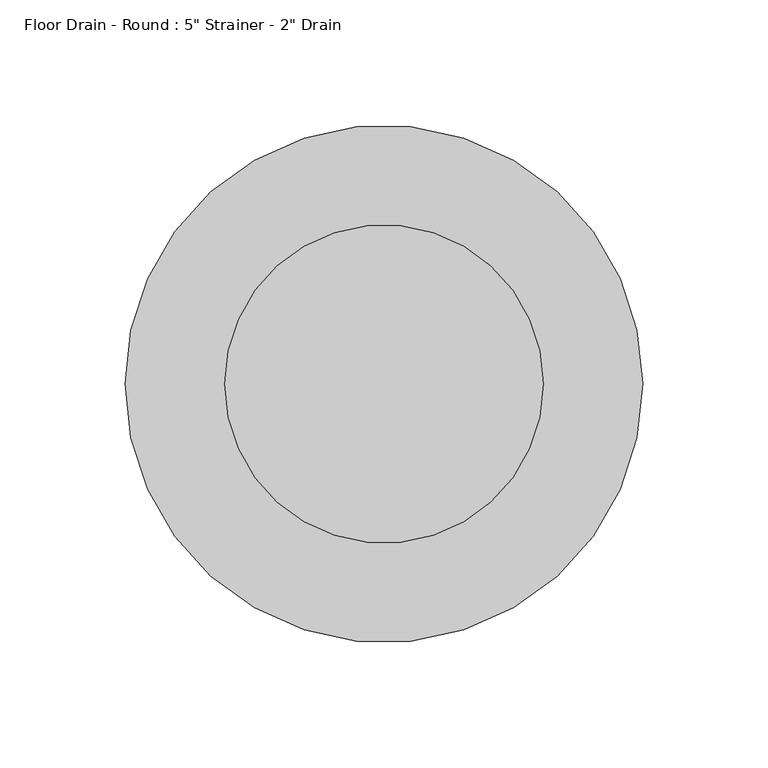
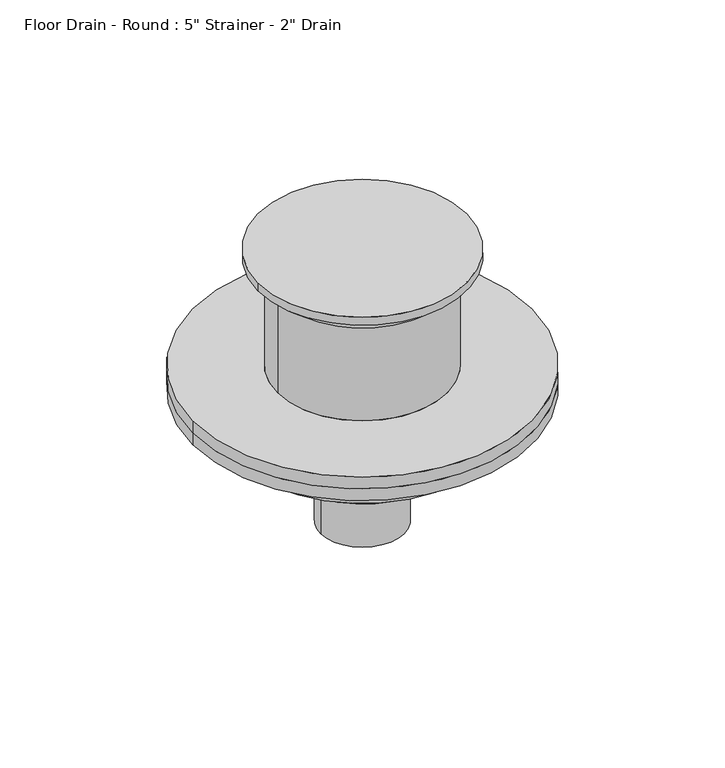
"""IFC4 building model written with IfcOpenShell, lengths in millimetres: flow terminal geometry."""

from ifc_helpers import new_model, si_unit, frame, origin, place, context, project, spatial, polyline, circle_curve, source, transform, mapped, element, save
from ifc_brep_helpers import plane_surface, cylinder_surface, revolved_surface, advanced_brep


def flow_terminal_accce45a(model_context):
    return source(origin(), model_context, "Body", "AdvancedBrep", [
        advanced_brep(
        [(103.1875, 0.0, -74.93), (-103.1875, 0.0, -74.93), (-51.59375, 0.0, -74.93), (51.59375, 0.0, -74.93), (103.1875, 0.0, -82.55), (-103.1875, 0.0, -82.55), (51.59375, 0.0, -15.24), (-51.59375, 0.0, -15.24), (-63.5, 0.0, -5.08), (63.5, 0.0, -5.08), (63.5, 0.0, 0.0), (-63.5, 0.0, 0.0)],
        [
            (0, 1, circle_curve(frame((0.0, 0.0, -74.93), z_axis=(0.0, 0.0, 1.0), x_axis=(-1.0, 0.0, 0.0)), 103.1875)),
            (1, 0, circle_curve(frame((0.0, 0.0, -74.93), z_axis=(0.0, 0.0, 1.0), x_axis=(-1.0, 0.0, 0.0)), 103.1875)),
            (2, 3, circle_curve(frame((0.0, 0.0, -74.93), z_axis=(0.0, 0.0, -1.0), x_axis=(-1.0, 0.0, 0.0)), 51.59375)),
            (3, 2, circle_curve(frame((0.0, 0.0, -74.93), z_axis=(0.0, 0.0, -1.0), x_axis=(-1.0, 0.0, 0.0)), 51.59375)),
            (4, 5, circle_curve(frame((0.0, 0.0, -82.55), z_axis=(0.0, 0.0, -1.0), x_axis=(-1.0, 0.0, 0.0)), 103.1875)),
            (5, 4, circle_curve(frame((0.0, 0.0, -82.55), z_axis=(0.0, 0.0, -1.0), x_axis=(-1.0, 0.0, 0.0)), 103.1875)),
            (0, 4),
            (5, 1),
            (6, 3),
            (2, 7),
            (7, 6, circle_curve(frame((0.0, 0.0, -15.24), z_axis=(0.0, 0.0, -1.0), x_axis=(-1.0, 0.0, 0.0)), 51.59375)),
            (6, 7, circle_curve(frame((0.0, 0.0, -15.24), z_axis=(0.0, 0.0, -1.0), x_axis=(-1.0, 0.0, 0.0)), 51.59375)),
            (7, 8),
            (8, 9, circle_curve(frame((0.0, 0.0, -5.08), z_axis=(0.0, 0.0, -1.0), x_axis=(-1.0, 0.0, 0.0)), 63.5)),
            (9, 6),
            (9, 8, circle_curve(frame((0.0, 0.0, -5.08), z_axis=(0.0, 0.0, -1.0), x_axis=(-1.0, 0.0, 0.0)), 63.5)),
            (10, 11, circle_curve(frame((0.0, 0.0, 0.0), z_axis=(0.0, 0.0, 1.0), x_axis=(-1.0, 0.0, 0.0)), 63.5)),
            (11, 10, circle_curve(frame((0.0, 0.0, 0.0), z_axis=(0.0, 0.0, 1.0), x_axis=(-1.0, 0.0, 0.0)), 63.5)),
            (10, 9),
            (8, 11),
        ],
        [
            plane_surface(frame((-103.1875, 0.0, -74.93), z_axis=(0.0, 0.0, 1.0), x_axis=(0.0, -1.0, 0.0))),
            plane_surface(frame((-103.1875, 0.0, -82.55), z_axis=(0.0, 0.0, -1.0), x_axis=(0.0, 1.0, 0.0))),
            cylinder_surface(frame((0.0, 0.0, -82.55), z_axis=(0.0, 0.0, 1.0), x_axis=(-1.0, 0.0, 0.0)), 103.1875),
            cylinder_surface(frame((0.0, 0.0, -74.93), z_axis=(0.0, 0.0, 1.0), x_axis=(-1.0, 0.0, 0.0)), 51.59375),
            revolved_surface(polyline([(-63.5, 0.0, -5.08), (-51.59375, 0.0, -15.24)]), (0.0, 0.0, 44.45), (0.0, 0.0, -1.0)),
            plane_surface(frame((-63.5, 0.0, 0.0), z_axis=(0.0, 0.0, 1.0), x_axis=(0.0, -1.0, 0.0))),
            cylinder_surface(frame((0.0, 0.0, -5.08), z_axis=(0.0, 0.0, 1.0), x_axis=(-1.0, 0.0, 0.0)), 63.5),
        ],
        [
            (0, [[1, 2], [3, 4]]),
            (1, [[5, 6]]),
            (2, [[-1, 7, -6, 8]]),
            (2, [[-2, -8, -5, -7]]),
            (3, [[9, -3, 10, 11]]),
            (3, [[-9, 12, -10, -4]]),
            (4, [[13, 14, 15, -11]]),
            (4, [[-13, -12, -15, 16]]),
            (5, [[17, 18]]),
            (6, [[-17, 19, -14, 20]]),
            (6, [[-18, -20, -16, -19]]),
        ],
    ),
        advanced_brep(
        [(25.4, 0.0, -174.625), (-25.4, 0.0, -174.625), (-25.4, 0.0, -128.5875), (25.4, 0.0, -128.5875), (51.3291667, 0.0, -128.5875), (-51.3291667, 0.0, -128.5875), (-51.3291667, 0.0, -110.1725), (51.3291667, 0.0, -110.1725), (77.2583333, 0.0, -110.1725), (-77.2583333, 0.0, -110.1725), (-77.2583333, 0.0, -90.17), (77.2583333, 0.0, -90.17), (103.1875, 0.0, -82.55), (-103.1875, 0.0, -82.55), (103.1875, 0.0, -90.17), (-103.1875, 0.0, -90.17)],
        [
            (0, 1, circle_curve(frame((0.0, 0.0, -174.625), z_axis=(0.0, 0.0, -1.0), x_axis=(-1.0, 0.0, 0.0)), 25.4)),
            (1, 0, circle_curve(frame((0.0, 0.0, -174.625), z_axis=(0.0, 0.0, -1.0), x_axis=(-1.0, 0.0, 0.0)), 25.4)),
            (1, 2),
            (2, 3, circle_curve(frame((0.0, 0.0, -128.5875), z_axis=(0.0, 0.0, -1.0), x_axis=(-1.0, 0.0, 0.0)), 25.4)),
            (3, 0),
            (3, 2, circle_curve(frame((0.0, 0.0, -128.5875), z_axis=(0.0, 0.0, -1.0), x_axis=(-1.0, 0.0, 0.0)), 25.4)),
            (4, 5, circle_curve(frame((0.0, 0.0, -128.5875), z_axis=(0.0, 0.0, -1.0), x_axis=(-1.0, 0.0, 0.0)), 51.3291667)),
            (5, 4, circle_curve(frame((0.0, 0.0, -128.5875), z_axis=(0.0, 0.0, -1.0), x_axis=(-1.0, 0.0, 0.0)), 51.3291667)),
            (5, 6),
            (6, 7, circle_curve(frame((0.0, 0.0, -110.1725), z_axis=(0.0, 0.0, -1.0), x_axis=(-1.0, 0.0, 0.0)), 51.3291667)),
            (7, 4),
            (7, 6, circle_curve(frame((0.0, 0.0, -110.1725), z_axis=(0.0, 0.0, -1.0), x_axis=(-1.0, 0.0, 0.0)), 51.3291667)),
            (8, 9, circle_curve(frame((0.0, 0.0, -110.1725), z_axis=(0.0, 0.0, -1.0), x_axis=(-1.0, 0.0, 0.0)), 77.2583333)),
            (9, 8, circle_curve(frame((0.0, 0.0, -110.1725), z_axis=(0.0, 0.0, -1.0), x_axis=(-1.0, 0.0, 0.0)), 77.2583333)),
            (9, 10),
            (10, 11, circle_curve(frame((0.0, 0.0, -90.17), z_axis=(0.0, 0.0, -1.0), x_axis=(-1.0, 0.0, 0.0)), 77.2583333)),
            (11, 8),
            (11, 10, circle_curve(frame((0.0, 0.0, -90.17), z_axis=(0.0, 0.0, -1.0), x_axis=(-1.0, 0.0, 0.0)), 77.2583333)),
            (12, 13, circle_curve(frame((0.0, 0.0, -82.55), z_axis=(0.0, 0.0, 1.0), x_axis=(-1.0, 0.0, 0.0)), 103.1875)),
            (13, 12, circle_curve(frame((0.0, 0.0, -82.55), z_axis=(0.0, 0.0, 1.0), x_axis=(-1.0, 0.0, 0.0)), 103.1875)),
            (14, 15, circle_curve(frame((0.0, 0.0, -90.17), z_axis=(0.0, 0.0, -1.0), x_axis=(-1.0, 0.0, 0.0)), 103.1875)),
            (15, 14, circle_curve(frame((0.0, 0.0, -90.17), z_axis=(0.0, 0.0, -1.0), x_axis=(-1.0, 0.0, 0.0)), 103.1875)),
            (12, 14),
            (15, 13),
        ],
        [
            plane_surface(frame((-25.4, 0.0, -174.625), z_axis=(0.0, 0.0, -1.0), x_axis=(0.0, 1.0, 0.0))),
            cylinder_surface(frame((0.0, 0.0, -174.625), z_axis=(0.0, 0.0, 1.0), x_axis=(-1.0, 0.0, 0.0)), 25.4),
            plane_surface(frame((-51.3291667, 0.0, -128.5875), z_axis=(0.0, 0.0, -1.0), x_axis=(0.0, 1.0, 0.0))),
            cylinder_surface(frame((0.0, 0.0, -128.5875), z_axis=(0.0, 0.0, 1.0), x_axis=(-1.0, 0.0, 0.0)), 51.3291667),
            plane_surface(frame((-77.2583333, 0.0, -110.1725), z_axis=(0.0, 0.0, -1.0), x_axis=(0.0, 1.0, 0.0))),
            cylinder_surface(frame((0.0, 0.0, -110.1725), z_axis=(0.0, 0.0, 1.0), x_axis=(-1.0, 0.0, 0.0)), 77.2583333),
            plane_surface(frame((-103.1875, 0.0, -82.55), z_axis=(0.0, 0.0, 1.0), x_axis=(0.0, -1.0, 0.0))),
            plane_surface(frame((-103.1875, 0.0, -90.17), z_axis=(0.0, 0.0, -1.0), x_axis=(0.0, 1.0, 0.0))),
            cylinder_surface(frame((0.0, 0.0, -90.17), z_axis=(0.0, 0.0, 1.0), x_axis=(-1.0, 0.0, 0.0)), 103.1875),
        ],
        [
            (0, [[1, 2]]),
            (1, [[-2, 3, 4, 5]]),
            (1, [[-1, -5, 6, -3]]),
            (2, [[7, 8], [-4, -6]]),
            (3, [[-8, 9, 10, 11]]),
            (3, [[-7, -11, 12, -9]]),
            (4, [[13, 14], [-10, -12]]),
            (5, [[-14, 15, 16, 17]]),
            (5, [[-13, -17, 18, -15]]),
            (6, [[19, 20]]),
            (7, [[21, 22], [-16, -18]]),
            (8, [[-19, 23, -22, 24]]),
            (8, [[-20, -24, -21, -23]]),
        ],
    ),
    ])


if __name__ == "__main__":
    model = new_model("IFC4")
    model_context = context("Model", 3, world=origin())
    ifc_project = project(units=[si_unit("LENGTHUNIT", "METRE", prefix="MILLI")], contexts=[model_context])
    site = spatial("IfcSite", under=ifc_project)
    building = spatial("IfcBuilding", under=site)
    placement = place(None, origin())
    flow_terminal_shape = flow_terminal_accce45a(model_context)
    element("IfcFlowTerminal", 1, ObjectType="Floor Drain - Round : 5\" Strainer - 2\" Drain", at=placement, inside=building, context=model_context, shape_type="MappedRepresentation", body=[
        mapped(flow_terminal_shape, transform((0.0, 0.0, 0.0), x_axis=(1.0, 0.0, 0.0), y_axis=(0.0, 1.0, 0.0), z_axis=(0.0, 0.0, 1.0))),
    ])
    save(model, "model.ifc")

# Revit data of these elements
# Type "Floor Drain - Round : 5\" Strainer - 2\" Drain"
#   WFU = 2
#   Strainer Height = 0' - 3 1/4"
#   Strainer Radius = 0' - 2 1/2"
#   Strainer Diameter = 0' - 5"
#   Radius 6 = 0' - 0 5/8"
#   Radius 5 = 0' - 1 1/4"
#   Radius 4 = 0' - 1 7/8"
#   Radius 2 = 0' - 3.04167"
#   Radius 1 = 0' - 2.02083"
#   Radius 3 = 0' - 2 1/32"
#   Pipe Radius = 1"
#   Pipe Diameter = 2"
#   Height 2 = 0' - 0.725"
#   Height 1 = 0' - 1 13/16"
#   Body Radius = 0' - 4 1/16"
#   Body Height = 0' - 3 5/8"
#   Body Diameter = 0' - 8 1/8"
#   Drain Material = none
#   HWFU = 0
#   Default Elevation = 0
#   CWFU = 0
